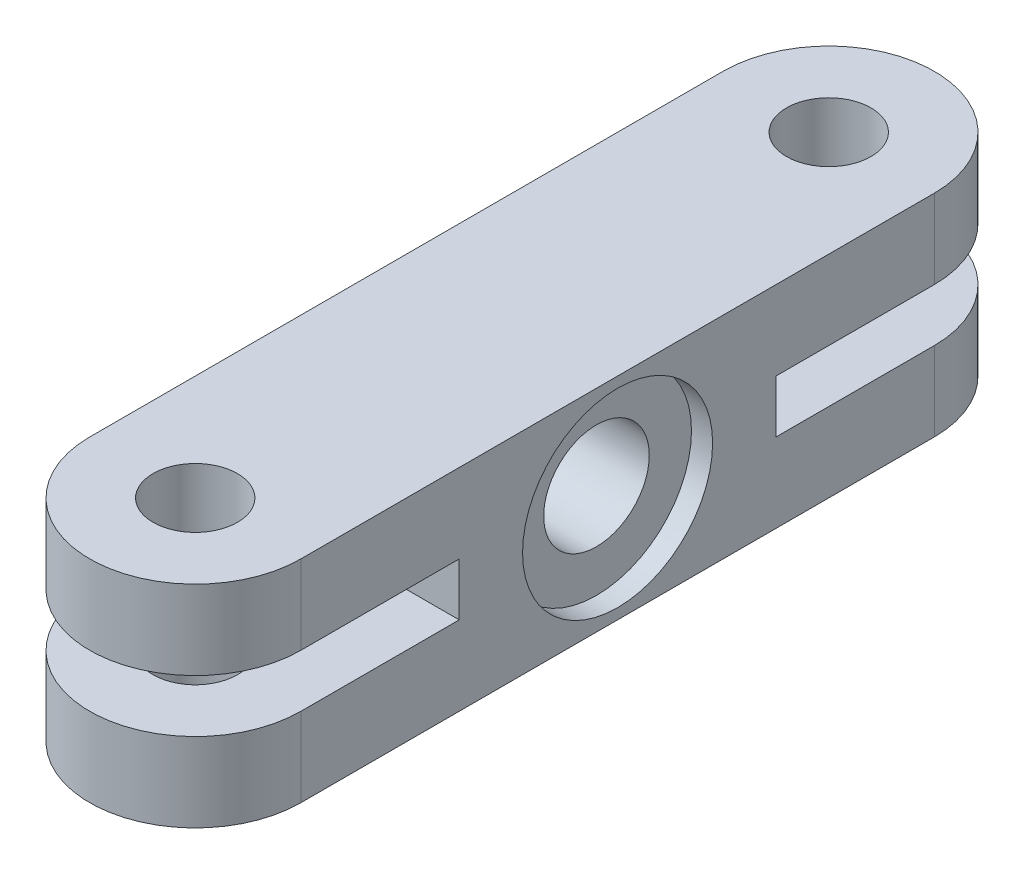
ISO-10303-21;
HEADER;
FILE_DESCRIPTION(('STEP AP214'),'2;1');
FILE_NAME('part.step','',(''),(''),'','','');
FILE_SCHEMA(('AUTOMOTIVE_DESIGN { 1 0 10303 214 1 1 1 1 }'));
ENDSEC;
DATA;
#1=APPLICATION_CONTEXT('core data for automotive mechanical design processes');
#2=APPLICATION_PROTOCOL_DEFINITION('international standard','automotive_design',2000,#1);
#3=PRODUCT_CONTEXT('',#1,'mechanical');
#4=PRODUCT('Part','Part','',(#3));
#5=PRODUCT_RELATED_PRODUCT_CATEGORY('part','',(#4));
#6=PRODUCT_DEFINITION_FORMATION('','',#4);
#7=PRODUCT_DEFINITION_CONTEXT('part definition',#1,'design');
#8=PRODUCT_DEFINITION('design','',#6,#7);
#9=PRODUCT_DEFINITION_SHAPE('','',#8);
#10=(LENGTH_UNIT() NAMED_UNIT(*) SI_UNIT(.MILLI.,.METRE.));
#11=(NAMED_UNIT(*) PLANE_ANGLE_UNIT() SI_UNIT($,.RADIAN.));
#12=(NAMED_UNIT(*) SI_UNIT($,.STERADIAN.) SOLID_ANGLE_UNIT());
#13=UNCERTAINTY_MEASURE_WITH_UNIT(LENGTH_MEASURE(1.E-05),#10,'distance_accuracy_value','');
#14=(GEOMETRIC_REPRESENTATION_CONTEXT(3) GLOBAL_UNCERTAINTY_ASSIGNED_CONTEXT((#13)) GLOBAL_UNIT_ASSIGNED_CONTEXT((#10,
#11,#12)) REPRESENTATION_CONTEXT('',''));
#15=CARTESIAN_POINT('',(0.,0.,0.));
#16=DIRECTION('',(0.,0.,1.));
#17=DIRECTION('',(1.,0.,0.));
#18=AXIS2_PLACEMENT_3D('',#15,#16,#17);
#19=CARTESIAN_POINT('',(-10.,0.,0.));
#20=DIRECTION('',(1.,0.,0.));
#21=DIRECTION('',(0.,0.,-1.));
#22=AXIS2_PLACEMENT_3D('',#19,#20,#21);
#23=CYLINDRICAL_SURFACE('',#22,5.);
#24=CARTESIAN_POINT('',(-10.,0.,0.));
#25=DIRECTION('',(1.,0.,0.));
#26=DIRECTION('',(0.,0.,-1.));
#27=AXIS2_PLACEMENT_3D('',#24,#25,#26);
#28=CIRCLE('',#27,5.);
#29=CARTESIAN_POINT('',(-10.,0.,-5.));
#30=VERTEX_POINT('',#29);
#31=EDGE_CURVE('E174',#30,#30,#28,.T.);
#32=ORIENTED_EDGE('',*,*,#31,.F.);
#33=EDGE_LOOP('',(#32));
#34=FACE_BOUND('',#33,.T.);
#35=CARTESIAN_POINT('',(8.00000000000001,0.,0.));
#36=DIRECTION('',(1.,0.,0.));
#37=DIRECTION('',(0.,0.,-1.));
#38=AXIS2_PLACEMENT_3D('',#35,#36,#37);
#39=CIRCLE('',#38,5.);
#40=CARTESIAN_POINT('',(8.00000000000001,0.,-5.));
#41=VERTEX_POINT('',#40);
#42=EDGE_CURVE('E44',#41,#41,#39,.F.);
#43=ORIENTED_EDGE('',*,*,#42,.F.);
#44=EDGE_LOOP('',(#43));
#45=FACE_BOUND('',#44,.T.);
#46=ADVANCED_FACE('F41',(#34,#45),#23,.F.);
#47=CARTESIAN_POINT('',(0.,10.,-30.));
#48=DIRECTION('',(0.,-1.,0.));
#49=DIRECTION('',(0.,0.,-1.));
#50=AXIS2_PLACEMENT_3D('',#47,#48,#49);
#51=CYLINDRICAL_SURFACE('',#50,10.);
#52=DIRECTION('',(0.,-1.,0.));
#53=VECTOR('',#52,1.);
#54=CARTESIAN_POINT('',(10.,10.,-30.));
#55=LINE('',#54,#53);
#56=CARTESIAN_POINT('',(10.,10.,-30.));
#57=VERTEX_POINT('',#56);
#58=CARTESIAN_POINT('',(10.,2.5,-30.));
#59=VERTEX_POINT('',#58);
#60=EDGE_CURVE('E233',#57,#59,#55,.T.);
#61=ORIENTED_EDGE('',*,*,#60,.T.);
#62=CARTESIAN_POINT('',(0.,2.5,-30.));
#63=DIRECTION('',(0.,1.,0.));
#64=DIRECTION('',(0.,0.,1.));
#65=AXIS2_PLACEMENT_3D('',#62,#63,#64);
#66=CIRCLE('',#65,10.);
#67=CARTESIAN_POINT('',(-10.,2.5,-30.));
#68=VERTEX_POINT('',#67);
#69=EDGE_CURVE('E195',#59,#68,#66,.T.);
#70=ORIENTED_EDGE('',*,*,#69,.T.);
#71=DIRECTION('',(0.,-1.,0.));
#72=VECTOR('',#71,1.);
#73=CARTESIAN_POINT('',(-10.,10.,-30.));
#74=LINE('',#73,#72);
#75=CARTESIAN_POINT('',(-10.,10.,-30.));
#76=VERTEX_POINT('',#75);
#77=EDGE_CURVE('E11',#76,#68,#74,.T.);
#78=ORIENTED_EDGE('',*,*,#77,.F.);
#79=CARTESIAN_POINT('',(0.,10.,-30.));
#80=DIRECTION('',(0.,1.,0.));
#81=DIRECTION('',(0.,0.,1.));
#82=AXIS2_PLACEMENT_3D('',#79,#80,#81);
#83=CIRCLE('',#82,10.);
#84=EDGE_CURVE('E212',#57,#76,#83,.T.);
#85=ORIENTED_EDGE('',*,*,#84,.F.);
#86=EDGE_LOOP('',(#61,#70,#78,#85));
#87=FACE_BOUND('',#86,.T.);
#88=ADVANCED_FACE('F275',(#87),#51,.T.);
#89=CARTESIAN_POINT('',(0.,10.,30.));
#90=DIRECTION('',(0.,-1.,0.));
#91=DIRECTION('',(0.,0.,-1.));
#92=AXIS2_PLACEMENT_3D('',#89,#90,#91);
#93=CYLINDRICAL_SURFACE('',#92,10.);
#94=DIRECTION('',(0.,-1.,0.));
#95=VECTOR('',#94,1.);
#96=CARTESIAN_POINT('',(-9.99999999999999,10.,30.));
#97=LINE('',#96,#95);
#98=CARTESIAN_POINT('',(-9.99999999999999,10.,30.));
#99=VERTEX_POINT('',#98);
#100=CARTESIAN_POINT('',(-10.,2.5,30.));
#101=VERTEX_POINT('',#100);
#102=EDGE_CURVE('E243',#99,#101,#97,.T.);
#103=ORIENTED_EDGE('',*,*,#102,.T.);
#104=CARTESIAN_POINT('',(0.,2.5,30.));
#105=DIRECTION('',(0.,1.,0.));
#106=DIRECTION('',(0.,0.,1.));
#107=AXIS2_PLACEMENT_3D('',#104,#105,#106);
#108=CIRCLE('',#107,10.);
#109=CARTESIAN_POINT('',(10.,2.5,30.));
#110=VERTEX_POINT('',#109);
#111=EDGE_CURVE('E196',#101,#110,#108,.T.);
#112=ORIENTED_EDGE('',*,*,#111,.T.);
#113=DIRECTION('',(0.,-1.,0.));
#114=VECTOR('',#113,1.);
#115=CARTESIAN_POINT('',(10.,10.,30.));
#116=LINE('',#115,#114);
#117=CARTESIAN_POINT('',(10.,10.,30.));
#118=VERTEX_POINT('',#117);
#119=EDGE_CURVE('E236',#118,#110,#116,.T.);
#120=ORIENTED_EDGE('',*,*,#119,.F.);
#121=CARTESIAN_POINT('',(0.,10.,30.));
#122=DIRECTION('',(0.,1.,0.));
#123=DIRECTION('',(0.,0.,1.));
#124=AXIS2_PLACEMENT_3D('',#121,#122,#123);
#125=CIRCLE('',#124,10.);
#126=EDGE_CURVE('E219',#99,#118,#125,.T.);
#127=ORIENTED_EDGE('',*,*,#126,.F.);
#128=EDGE_LOOP('',(#103,#112,#120,#127));
#129=FACE_BOUND('',#128,.T.);
#130=ADVANCED_FACE('F263',(#129),#93,.T.);
#131=CARTESIAN_POINT('',(0.,-10.,30.));
#132=DIRECTION('',(0.,1.,0.));
#133=DIRECTION('',(0.,0.,1.));
#134=AXIS2_PLACEMENT_3D('',#131,#132,#133);
#135=CYLINDRICAL_SURFACE('',#134,4.);
#136=CARTESIAN_POINT('',(0.,2.5,30.));
#137=DIRECTION('',(0.,1.,0.));
#138=DIRECTION('',(0.,0.,1.));
#139=AXIS2_PLACEMENT_3D('',#136,#137,#138);
#140=CIRCLE('',#139,4.);
#141=CARTESIAN_POINT('',(0.,2.5,34.));
#142=VERTEX_POINT('',#141);
#143=EDGE_CURVE('E197',#142,#142,#140,.F.);
#144=ORIENTED_EDGE('',*,*,#143,.T.);
#145=EDGE_LOOP('',(#144));
#146=FACE_BOUND('',#145,.T.);
#147=CARTESIAN_POINT('',(0.,10.,30.));
#148=DIRECTION('',(0.,1.,0.));
#149=DIRECTION('',(0.,0.,1.));
#150=AXIS2_PLACEMENT_3D('',#147,#148,#149);
#151=CIRCLE('',#150,4.);
#152=CARTESIAN_POINT('',(0.,10.,34.));
#153=VERTEX_POINT('',#152);
#154=EDGE_CURVE('E207',#153,#153,#151,.T.);
#155=ORIENTED_EDGE('',*,*,#154,.T.);
#156=EDGE_LOOP('',(#155));
#157=FACE_BOUND('',#156,.T.);
#158=ADVANCED_FACE('F252',(#146,#157),#135,.F.);
#159=CARTESIAN_POINT('',(0.,-10.,-30.));
#160=DIRECTION('',(0.,1.,0.));
#161=DIRECTION('',(0.,0.,1.));
#162=AXIS2_PLACEMENT_3D('',#159,#160,#161);
#163=CYLINDRICAL_SURFACE('',#162,4.);
#164=CARTESIAN_POINT('',(0.,2.5,-30.));
#165=DIRECTION('',(0.,1.,0.));
#166=DIRECTION('',(0.,0.,1.));
#167=AXIS2_PLACEMENT_3D('',#164,#165,#166);
#168=CIRCLE('',#167,4.);
#169=CARTESIAN_POINT('',(0.,2.5,-26.));
#170=VERTEX_POINT('',#169);
#171=EDGE_CURVE('E191',#170,#170,#168,.F.);
#172=ORIENTED_EDGE('',*,*,#171,.T.);
#173=EDGE_LOOP('',(#172));
#174=FACE_BOUND('',#173,.T.);
#175=CARTESIAN_POINT('',(0.,10.,-30.));
#176=DIRECTION('',(0.,1.,0.));
#177=DIRECTION('',(0.,0.,1.));
#178=AXIS2_PLACEMENT_3D('',#175,#176,#177);
#179=CIRCLE('',#178,4.);
#180=CARTESIAN_POINT('',(0.,10.,-26.));
#181=VERTEX_POINT('',#180);
#182=EDGE_CURVE('E206',#181,#181,#179,.T.);
#183=ORIENTED_EDGE('',*,*,#182,.T.);
#184=EDGE_LOOP('',(#183));
#185=FACE_BOUND('',#184,.T.);
#186=ADVANCED_FACE('F323',(#174,#185),#163,.F.);
#187=CARTESIAN_POINT('',(-10.,-2.5,-30.));
#188=VERTEX_POINT('',#187);
#189=CARTESIAN_POINT('',(-10.,-10.,-30.));
#190=VERTEX_POINT('',#189);
#191=EDGE_CURVE('E49',#188,#190,#74,.T.);
#192=ORIENTED_EDGE('',*,*,#191,.F.);
#193=CARTESIAN_POINT('',(0.,-2.5,-30.));
#194=DIRECTION('',(0.,-1.,0.));
#195=DIRECTION('',(0.,0.,-1.));
#196=AXIS2_PLACEMENT_3D('',#193,#194,#195);
#197=CIRCLE('',#196,10.);
#198=CARTESIAN_POINT('',(10.,-2.5,-30.));
#199=VERTEX_POINT('',#198);
#200=EDGE_CURVE('E187',#188,#199,#197,.T.);
#201=ORIENTED_EDGE('',*,*,#200,.T.);
#202=CARTESIAN_POINT('',(10.,-10.,-30.));
#203=VERTEX_POINT('',#202);
#204=EDGE_CURVE('E221',#199,#203,#55,.T.);
#205=ORIENTED_EDGE('',*,*,#204,.T.);
#206=CARTESIAN_POINT('',(0.,-10.,-30.));
#207=DIRECTION('',(0.,1.,0.));
#208=DIRECTION('',(0.,0.,1.));
#209=AXIS2_PLACEMENT_3D('',#206,#207,#208);
#210=CIRCLE('',#209,10.);
#211=EDGE_CURVE('E202',#203,#190,#210,.T.);
#212=ORIENTED_EDGE('',*,*,#211,.T.);
#213=EDGE_LOOP('',(#192,#201,#205,#212));
#214=FACE_BOUND('',#213,.T.);
#215=ADVANCED_FACE('F43',(#214),#51,.T.);
#216=CARTESIAN_POINT('',(-10.,10.,-30.));
#217=DIRECTION('',(1.,0.,0.));
#218=DIRECTION('',(0.,0.,-1.));
#219=AXIS2_PLACEMENT_3D('',#216,#217,#218);
#220=PLANE('',#219);
#221=ORIENTED_EDGE('',*,*,#31,.T.);
#222=EDGE_LOOP('',(#221));
#223=FACE_BOUND('',#222,.T.);
#224=DIRECTION('',(0.,1.,0.));
#225=VECTOR('',#224,1.);
#226=CARTESIAN_POINT('',(-10.,2.5,15.));
#227=LINE('',#226,#225);
#228=CARTESIAN_POINT('',(-10.,-2.5,15.));
#229=VERTEX_POINT('',#228);
#230=CARTESIAN_POINT('',(-10.,2.5,15.));
#231=VERTEX_POINT('',#230);
#232=EDGE_CURVE('E145',#229,#231,#227,.T.);
#233=ORIENTED_EDGE('',*,*,#232,.T.);
#234=DIRECTION('',(0.,0.,1.));
#235=VECTOR('',#234,1.);
#236=CARTESIAN_POINT('',(-10.,2.5,45.7528109702023));
#237=LINE('',#236,#235);
#238=EDGE_CURVE('E143',#231,#101,#237,.T.);
#239=ORIENTED_EDGE('',*,*,#238,.T.);
#240=ORIENTED_EDGE('',*,*,#102,.F.);
#241=DIRECTION('',(0.,0.,1.));
#242=VECTOR('',#241,1.);
#243=CARTESIAN_POINT('',(-10.,10.,-30.));
#244=LINE('',#243,#242);
#245=EDGE_CURVE('E220',#76,#99,#244,.T.);
#246=ORIENTED_EDGE('',*,*,#245,.F.);
#247=ORIENTED_EDGE('',*,*,#77,.T.);
#248=DIRECTION('',(0.,0.,1.));
#249=VECTOR('',#248,1.);
#250=CARTESIAN_POINT('',(-10.,2.5,-15.));
#251=LINE('',#250,#249);
#252=CARTESIAN_POINT('',(-10.,2.5,-15.));
#253=VERTEX_POINT('',#252);
#254=EDGE_CURVE('E166',#68,#253,#251,.T.);
#255=ORIENTED_EDGE('',*,*,#254,.T.);
#256=DIRECTION('',(0.,-1.,0.));
#257=VECTOR('',#256,1.);
#258=CARTESIAN_POINT('',(-10.,2.5,-15.));
#259=LINE('',#258,#257);
#260=CARTESIAN_POINT('',(-10.,-2.5,-15.));
#261=VERTEX_POINT('',#260);
#262=EDGE_CURVE('E176',#253,#261,#259,.T.);
#263=ORIENTED_EDGE('',*,*,#262,.T.);
#264=DIRECTION('',(0.,0.,-1.));
#265=VECTOR('',#264,1.);
#266=CARTESIAN_POINT('',(-10.,-2.5,-15.));
#267=LINE('',#266,#265);
#268=EDGE_CURVE('E182',#261,#188,#267,.T.);
#269=ORIENTED_EDGE('',*,*,#268,.T.);
#270=ORIENTED_EDGE('',*,*,#191,.T.);
#271=DIRECTION('',(0.,0.,1.));
#272=VECTOR('',#271,1.);
#273=CARTESIAN_POINT('',(-10.,-10.,-30.));
#274=LINE('',#273,#272);
#275=CARTESIAN_POINT('',(-9.99999999999999,-10.,30.));
#276=VERTEX_POINT('',#275);
#277=EDGE_CURVE('E229',#190,#276,#274,.T.);
#278=ORIENTED_EDGE('',*,*,#277,.T.);
#279=CARTESIAN_POINT('',(-10.,-2.5,30.));
#280=VERTEX_POINT('',#279);
#281=EDGE_CURVE('E153',#280,#276,#97,.T.);
#282=ORIENTED_EDGE('',*,*,#281,.F.);
#283=DIRECTION('',(0.,0.,-1.));
#284=VECTOR('',#283,1.);
#285=CARTESIAN_POINT('',(-10.,-2.5,45.7528109702023));
#286=LINE('',#285,#284);
#287=EDGE_CURVE('E131',#280,#229,#286,.T.);
#288=ORIENTED_EDGE('',*,*,#287,.T.);
#289=EDGE_LOOP('',(#233,#239,#240,#246,#247,#255,#263,#269,#270,#278,#282,#288));
#290=FACE_BOUND('',#289,.T.);
#291=ADVANCED_FACE('F151',(#223,#290),#220,.F.);
#292=CARTESIAN_POINT('',(10.,-2.5,30.));
#293=VERTEX_POINT('',#292);
#294=CARTESIAN_POINT('',(10.,-10.,30.));
#295=VERTEX_POINT('',#294);
#296=EDGE_CURVE('E240',#293,#295,#116,.T.);
#297=ORIENTED_EDGE('',*,*,#296,.F.);
#298=CARTESIAN_POINT('',(0.,-2.5,30.));
#299=DIRECTION('',(0.,-1.,0.));
#300=DIRECTION('',(0.,0.,-1.));
#301=AXIS2_PLACEMENT_3D('',#298,#299,#300);
#302=CIRCLE('',#301,10.);
#303=EDGE_CURVE('E66',#293,#280,#302,.T.);
#304=ORIENTED_EDGE('',*,*,#303,.T.);
#305=ORIENTED_EDGE('',*,*,#281,.T.);
#306=CARTESIAN_POINT('',(0.,-10.,30.));
#307=DIRECTION('',(0.,1.,0.));
#308=DIRECTION('',(0.,0.,1.));
#309=AXIS2_PLACEMENT_3D('',#306,#307,#308);
#310=CIRCLE('',#309,10.);
#311=EDGE_CURVE('E230',#276,#295,#310,.T.);
#312=ORIENTED_EDGE('',*,*,#311,.T.);
#313=EDGE_LOOP('',(#297,#304,#305,#312));
#314=FACE_BOUND('',#313,.T.);
#315=ADVANCED_FACE('F291',(#314),#93,.T.);
#316=CARTESIAN_POINT('',(10.,10.,-30.));
#317=DIRECTION('',(-1.,0.,0.));
#318=DIRECTION('',(0.,0.,1.));
#319=AXIS2_PLACEMENT_3D('',#316,#317,#318);
#320=PLANE('',#319);
#321=CARTESIAN_POINT('',(10.,0.,0.));
#322=DIRECTION('',(1.,0.,0.));
#323=DIRECTION('',(0.,0.,-1.));
#324=AXIS2_PLACEMENT_3D('',#321,#322,#323);
#325=CIRCLE('',#324,9.);
#326=CARTESIAN_POINT('',(10.,0.,-9.));
#327=VERTEX_POINT('',#326);
#328=EDGE_CURVE('E157',#327,#327,#325,.T.);
#329=ORIENTED_EDGE('',*,*,#328,.F.);
#330=EDGE_LOOP('',(#329));
#331=FACE_BOUND('',#330,.T.);
#332=ORIENTED_EDGE('',*,*,#119,.T.);
#333=DIRECTION('',(0.,0.,1.));
#334=VECTOR('',#333,1.);
#335=CARTESIAN_POINT('',(10.,2.5,45.7528109702023));
#336=LINE('',#335,#334);
#337=CARTESIAN_POINT('',(10.,2.5,15.));
#338=VERTEX_POINT('',#337);
#339=EDGE_CURVE('E152',#338,#110,#336,.T.);
#340=ORIENTED_EDGE('',*,*,#339,.F.);
#341=DIRECTION('',(0.,1.,0.));
#342=VECTOR('',#341,1.);
#343=CARTESIAN_POINT('',(10.,2.5,15.));
#344=LINE('',#343,#342);
#345=CARTESIAN_POINT('',(10.,-2.5,15.));
#346=VERTEX_POINT('',#345);
#347=EDGE_CURVE('E156',#346,#338,#344,.T.);
#348=ORIENTED_EDGE('',*,*,#347,.F.);
#349=DIRECTION('',(0.,0.,-1.));
#350=VECTOR('',#349,1.);
#351=CARTESIAN_POINT('',(10.,-2.5,45.7528109702023));
#352=LINE('',#351,#350);
#353=EDGE_CURVE('E136',#293,#346,#352,.T.);
#354=ORIENTED_EDGE('',*,*,#353,.F.);
#355=ORIENTED_EDGE('',*,*,#296,.T.);
#356=DIRECTION('',(0.,0.,-1.));
#357=VECTOR('',#356,1.);
#358=CARTESIAN_POINT('',(10.,-10.,-30.));
#359=LINE('',#358,#357);
#360=EDGE_CURVE('E217',#295,#203,#359,.T.);
#361=ORIENTED_EDGE('',*,*,#360,.T.);
#362=ORIENTED_EDGE('',*,*,#204,.F.);
#363=DIRECTION('',(0.,0.,-1.));
#364=VECTOR('',#363,1.);
#365=CARTESIAN_POINT('',(10.,-2.5,-15.));
#366=LINE('',#365,#364);
#367=CARTESIAN_POINT('',(10.,-2.5,-15.));
#368=VERTEX_POINT('',#367);
#369=EDGE_CURVE('E171',#368,#199,#366,.T.);
#370=ORIENTED_EDGE('',*,*,#369,.F.);
#371=DIRECTION('',(0.,-1.,0.));
#372=VECTOR('',#371,1.);
#373=CARTESIAN_POINT('',(10.,2.5,-15.));
#374=LINE('',#373,#372);
#375=CARTESIAN_POINT('',(10.,2.5,-15.));
#376=VERTEX_POINT('',#375);
#377=EDGE_CURVE('E59',#376,#368,#374,.T.);
#378=ORIENTED_EDGE('',*,*,#377,.F.);
#379=DIRECTION('',(0.,0.,1.));
#380=VECTOR('',#379,1.);
#381=CARTESIAN_POINT('',(10.,2.5,-15.));
#382=LINE('',#381,#380);
#383=EDGE_CURVE('E172',#59,#376,#382,.T.);
#384=ORIENTED_EDGE('',*,*,#383,.F.);
#385=ORIENTED_EDGE('',*,*,#60,.F.);
#386=DIRECTION('',(0.,0.,-1.));
#387=VECTOR('',#386,1.);
#388=CARTESIAN_POINT('',(10.,10.,-30.));
#389=LINE('',#388,#387);
#390=EDGE_CURVE('E225',#118,#57,#389,.T.);
#391=ORIENTED_EDGE('',*,*,#390,.F.);
#392=EDGE_LOOP('',(#332,#340,#348,#354,#355,#361,#362,#370,#378,#384,#385,#391));
#393=FACE_BOUND('',#392,.T.);
#394=ADVANCED_FACE('F280',(#331,#393),#320,.F.);
#395=CARTESIAN_POINT('',(0.,10.,-30.));
#396=DIRECTION('',(0.,1.,0.));
#397=DIRECTION('',(0.,0.,1.));
#398=AXIS2_PLACEMENT_3D('',#395,#396,#397);
#399=PLANE('',#398);
#400=ORIENTED_EDGE('',*,*,#182,.F.);
#401=EDGE_LOOP('',(#400));
#402=FACE_BOUND('',#401,.T.);
#403=ORIENTED_EDGE('',*,*,#154,.F.);
#404=EDGE_LOOP('',(#403));
#405=FACE_BOUND('',#404,.T.);
#406=ORIENTED_EDGE('',*,*,#84,.T.);
#407=ORIENTED_EDGE('',*,*,#245,.T.);
#408=ORIENTED_EDGE('',*,*,#126,.T.);
#409=ORIENTED_EDGE('',*,*,#390,.T.);
#410=EDGE_LOOP('',(#406,#407,#408,#409));
#411=FACE_BOUND('',#410,.T.);
#412=ADVANCED_FACE('F270',(#402,#405,#411),#399,.T.);
#413=CARTESIAN_POINT('',(0.,-10.,-30.));
#414=DIRECTION('',(0.,1.,0.));
#415=DIRECTION('',(0.,0.,1.));
#416=AXIS2_PLACEMENT_3D('',#413,#414,#415);
#417=PLANE('',#416);
#418=CARTESIAN_POINT('',(0.,-10.,-30.));
#419=DIRECTION('',(0.,1.,0.));
#420=DIRECTION('',(0.,0.,1.));
#421=AXIS2_PLACEMENT_3D('',#418,#419,#420);
#422=CIRCLE('',#421,4.);
#423=CARTESIAN_POINT('',(0.,-10.,-26.));
#424=VERTEX_POINT('',#423);
#425=EDGE_CURVE('E205',#424,#424,#422,.T.);
#426=ORIENTED_EDGE('',*,*,#425,.T.);
#427=EDGE_LOOP('',(#426));
#428=FACE_BOUND('',#427,.T.);
#429=CARTESIAN_POINT('',(0.,-10.,30.));
#430=DIRECTION('',(0.,1.,0.));
#431=DIRECTION('',(0.,0.,1.));
#432=AXIS2_PLACEMENT_3D('',#429,#430,#431);
#433=CIRCLE('',#432,4.);
#434=CARTESIAN_POINT('',(0.,-10.,34.));
#435=VERTEX_POINT('',#434);
#436=EDGE_CURVE('E203',#435,#435,#433,.T.);
#437=ORIENTED_EDGE('',*,*,#436,.T.);
#438=EDGE_LOOP('',(#437));
#439=FACE_BOUND('',#438,.T.);
#440=ORIENTED_EDGE('',*,*,#211,.F.);
#441=ORIENTED_EDGE('',*,*,#360,.F.);
#442=ORIENTED_EDGE('',*,*,#311,.F.);
#443=ORIENTED_EDGE('',*,*,#277,.F.);
#444=EDGE_LOOP('',(#440,#441,#442,#443));
#445=FACE_BOUND('',#444,.T.);
#446=ADVANCED_FACE('F288',(#428,#439,#445),#417,.F.);
#447=CARTESIAN_POINT('',(0.,-2.5,30.));
#448=DIRECTION('',(0.,-1.,0.));
#449=DIRECTION('',(0.,0.,-1.));
#450=AXIS2_PLACEMENT_3D('',#447,#448,#449);
#451=CIRCLE('',#450,4.);
#452=CARTESIAN_POINT('',(0.,-2.5,26.));
#453=VERTEX_POINT('',#452);
#454=EDGE_CURVE('E194',#453,#453,#451,.F.);
#455=ORIENTED_EDGE('',*,*,#454,.T.);
#456=EDGE_LOOP('',(#455));
#457=FACE_BOUND('',#456,.T.);
#458=ORIENTED_EDGE('',*,*,#436,.F.);
#459=EDGE_LOOP('',(#458));
#460=FACE_BOUND('',#459,.T.);
#461=ADVANCED_FACE('F321',(#457,#460),#135,.F.);
#462=CARTESIAN_POINT('',(0.,-2.5,-30.));
#463=DIRECTION('',(0.,-1.,0.));
#464=DIRECTION('',(0.,0.,-1.));
#465=AXIS2_PLACEMENT_3D('',#462,#463,#464);
#466=CIRCLE('',#465,4.);
#467=CARTESIAN_POINT('',(0.,-2.5,-34.));
#468=VERTEX_POINT('',#467);
#469=EDGE_CURVE('E164',#468,#468,#466,.F.);
#470=ORIENTED_EDGE('',*,*,#469,.T.);
#471=EDGE_LOOP('',(#470));
#472=FACE_BOUND('',#471,.T.);
#473=ORIENTED_EDGE('',*,*,#425,.F.);
#474=EDGE_LOOP('',(#473));
#475=FACE_BOUND('',#474,.T.);
#476=ADVANCED_FACE('F318',(#472,#475),#163,.F.);
#477=CARTESIAN_POINT('',(-10.,2.5,-15.));
#478=DIRECTION('',(0.,1.,0.));
#479=DIRECTION('',(0.,0.,1.));
#480=AXIS2_PLACEMENT_3D('',#477,#478,#479);
#481=PLANE('',#480);
#482=ORIENTED_EDGE('',*,*,#171,.F.);
#483=EDGE_LOOP('',(#482));
#484=FACE_BOUND('',#483,.T.);
#485=ORIENTED_EDGE('',*,*,#383,.T.);
#486=DIRECTION('',(1.,0.,0.));
#487=VECTOR('',#486,1.);
#488=CARTESIAN_POINT('',(-10.,2.5,-15.));
#489=LINE('',#488,#487);
#490=EDGE_CURVE('E168',#253,#376,#489,.T.);
#491=ORIENTED_EDGE('',*,*,#490,.F.);
#492=ORIENTED_EDGE('',*,*,#254,.F.);
#493=ORIENTED_EDGE('',*,*,#69,.F.);
#494=EDGE_LOOP('',(#485,#491,#492,#493));
#495=FACE_BOUND('',#494,.T.);
#496=ADVANCED_FACE('F274',(#484,#495),#481,.F.);
#497=CARTESIAN_POINT('',(-10.,-2.5,-15.));
#498=DIRECTION('',(0.,-1.,0.));
#499=DIRECTION('',(0.,0.,-1.));
#500=AXIS2_PLACEMENT_3D('',#497,#498,#499);
#501=PLANE('',#500);
#502=ORIENTED_EDGE('',*,*,#469,.F.);
#503=EDGE_LOOP('',(#502));
#504=FACE_BOUND('',#503,.T.);
#505=ORIENTED_EDGE('',*,*,#268,.F.);
#506=DIRECTION('',(1.,0.,0.));
#507=VECTOR('',#506,1.);
#508=CARTESIAN_POINT('',(-10.,-2.5,-15.));
#509=LINE('',#508,#507);
#510=EDGE_CURVE('E170',#261,#368,#509,.T.);
#511=ORIENTED_EDGE('',*,*,#510,.T.);
#512=ORIENTED_EDGE('',*,*,#369,.T.);
#513=ORIENTED_EDGE('',*,*,#200,.F.);
#514=EDGE_LOOP('',(#505,#511,#512,#513));
#515=FACE_BOUND('',#514,.T.);
#516=ADVANCED_FACE('F284',(#504,#515),#501,.F.);
#517=CARTESIAN_POINT('',(-10.,2.5,-15.));
#518=DIRECTION('',(0.,0.,1.));
#519=DIRECTION('',(1.,0.,0.));
#520=AXIS2_PLACEMENT_3D('',#517,#518,#519);
#521=PLANE('',#520);
#522=ORIENTED_EDGE('',*,*,#377,.T.);
#523=ORIENTED_EDGE('',*,*,#510,.F.);
#524=ORIENTED_EDGE('',*,*,#262,.F.);
#525=ORIENTED_EDGE('',*,*,#490,.T.);
#526=EDGE_LOOP('',(#522,#523,#524,#525));
#527=FACE_BOUND('',#526,.T.);
#528=ADVANCED_FACE('F256',(#527),#521,.F.);
#529=CARTESIAN_POINT('',(-10.,2.5,45.7528109702023));
#530=DIRECTION('',(0.,1.,0.));
#531=DIRECTION('',(0.,0.,1.));
#532=AXIS2_PLACEMENT_3D('',#529,#530,#531);
#533=PLANE('',#532);
#534=ORIENTED_EDGE('',*,*,#143,.F.);
#535=EDGE_LOOP('',(#534));
#536=FACE_BOUND('',#535,.T.);
#537=ORIENTED_EDGE('',*,*,#238,.F.);
#538=DIRECTION('',(1.,0.,0.));
#539=VECTOR('',#538,1.);
#540=CARTESIAN_POINT('',(-10.,2.5,15.));
#541=LINE('',#540,#539);
#542=EDGE_CURVE('E139',#231,#338,#541,.T.);
#543=ORIENTED_EDGE('',*,*,#542,.T.);
#544=ORIENTED_EDGE('',*,*,#339,.T.);
#545=ORIENTED_EDGE('',*,*,#111,.F.);
#546=EDGE_LOOP('',(#537,#543,#544,#545));
#547=FACE_BOUND('',#546,.T.);
#548=ADVANCED_FACE('F254',(#536,#547),#533,.F.);
#549=CARTESIAN_POINT('',(-10.,-2.5,45.7528109702023));
#550=DIRECTION('',(0.,-1.,0.));
#551=DIRECTION('',(0.,0.,-1.));
#552=AXIS2_PLACEMENT_3D('',#549,#550,#551);
#553=PLANE('',#552);
#554=ORIENTED_EDGE('',*,*,#454,.F.);
#555=EDGE_LOOP('',(#554));
#556=FACE_BOUND('',#555,.T.);
#557=ORIENTED_EDGE('',*,*,#353,.T.);
#558=DIRECTION('',(1.,0.,0.));
#559=VECTOR('',#558,1.);
#560=CARTESIAN_POINT('',(-10.,-2.5,15.));
#561=LINE('',#560,#559);
#562=EDGE_CURVE('E133',#229,#346,#561,.T.);
#563=ORIENTED_EDGE('',*,*,#562,.F.);
#564=ORIENTED_EDGE('',*,*,#287,.F.);
#565=ORIENTED_EDGE('',*,*,#303,.F.);
#566=EDGE_LOOP('',(#557,#563,#564,#565));
#567=FACE_BOUND('',#566,.T.);
#568=ADVANCED_FACE('F132',(#556,#567),#553,.F.);
#569=CARTESIAN_POINT('',(-10.,2.5,15.));
#570=DIRECTION('',(0.,0.,-1.));
#571=DIRECTION('',(-1.,0.,0.));
#572=AXIS2_PLACEMENT_3D('',#569,#570,#571);
#573=PLANE('',#572);
#574=ORIENTED_EDGE('',*,*,#347,.T.);
#575=ORIENTED_EDGE('',*,*,#542,.F.);
#576=ORIENTED_EDGE('',*,*,#232,.F.);
#577=ORIENTED_EDGE('',*,*,#562,.T.);
#578=EDGE_LOOP('',(#574,#575,#576,#577));
#579=FACE_BOUND('',#578,.T.);
#580=ADVANCED_FACE('F144',(#579),#573,.F.);
#581=CARTESIAN_POINT('',(8.00000000000001,0.,0.));
#582=DIRECTION('',(1.,0.,0.));
#583=DIRECTION('',(0.,0.,-1.));
#584=AXIS2_PLACEMENT_3D('',#581,#582,#583);
#585=PLANE('',#584);
#586=CARTESIAN_POINT('',(8.00000000000001,0.,0.));
#587=DIRECTION('',(1.,0.,0.));
#588=DIRECTION('',(0.,0.,-1.));
#589=AXIS2_PLACEMENT_3D('',#586,#587,#588);
#590=CIRCLE('',#589,9.);
#591=CARTESIAN_POINT('',(8.00000000000001,0.,-9.));
#592=VERTEX_POINT('',#591);
#593=EDGE_CURVE('E481',#592,#592,#590,.T.);
#594=ORIENTED_EDGE('',*,*,#593,.T.);
#595=EDGE_LOOP('',(#594));
#596=FACE_BOUND('',#595,.T.);
#597=ORIENTED_EDGE('',*,*,#42,.T.);
#598=EDGE_LOOP('',(#597));
#599=FACE_BOUND('',#598,.T.);
#600=ADVANCED_FACE('F452',(#596,#599),#585,.T.);
#601=CARTESIAN_POINT('',(8.00000000000001,0.,0.));
#602=DIRECTION('',(1.,0.,0.));
#603=DIRECTION('',(0.,0.,-1.));
#604=AXIS2_PLACEMENT_3D('',#601,#602,#603);
#605=CYLINDRICAL_SURFACE('',#604,9.);
#606=ORIENTED_EDGE('',*,*,#593,.F.);
#607=EDGE_LOOP('',(#606));
#608=FACE_BOUND('',#607,.T.);
#609=ORIENTED_EDGE('',*,*,#328,.T.);
#610=EDGE_LOOP('',(#609));
#611=FACE_BOUND('',#610,.T.);
#612=ADVANCED_FACE('F461',(#608,#611),#605,.F.);
#613=CLOSED_SHELL('',(#46,#88,#130,#158,#186,#215,#291,#315,#394,#412,#446,#461,#476,#496,#516,
#528,#548,#568,#580,#600,#612));
#614=MANIFOLD_SOLID_BREP('B2',#613);
#615=ADVANCED_BREP_SHAPE_REPRESENTATION('',(#18,#614),#14);
#616=SHAPE_DEFINITION_REPRESENTATION(#9,#615);
ENDSEC;
END-ISO-10303-21;
